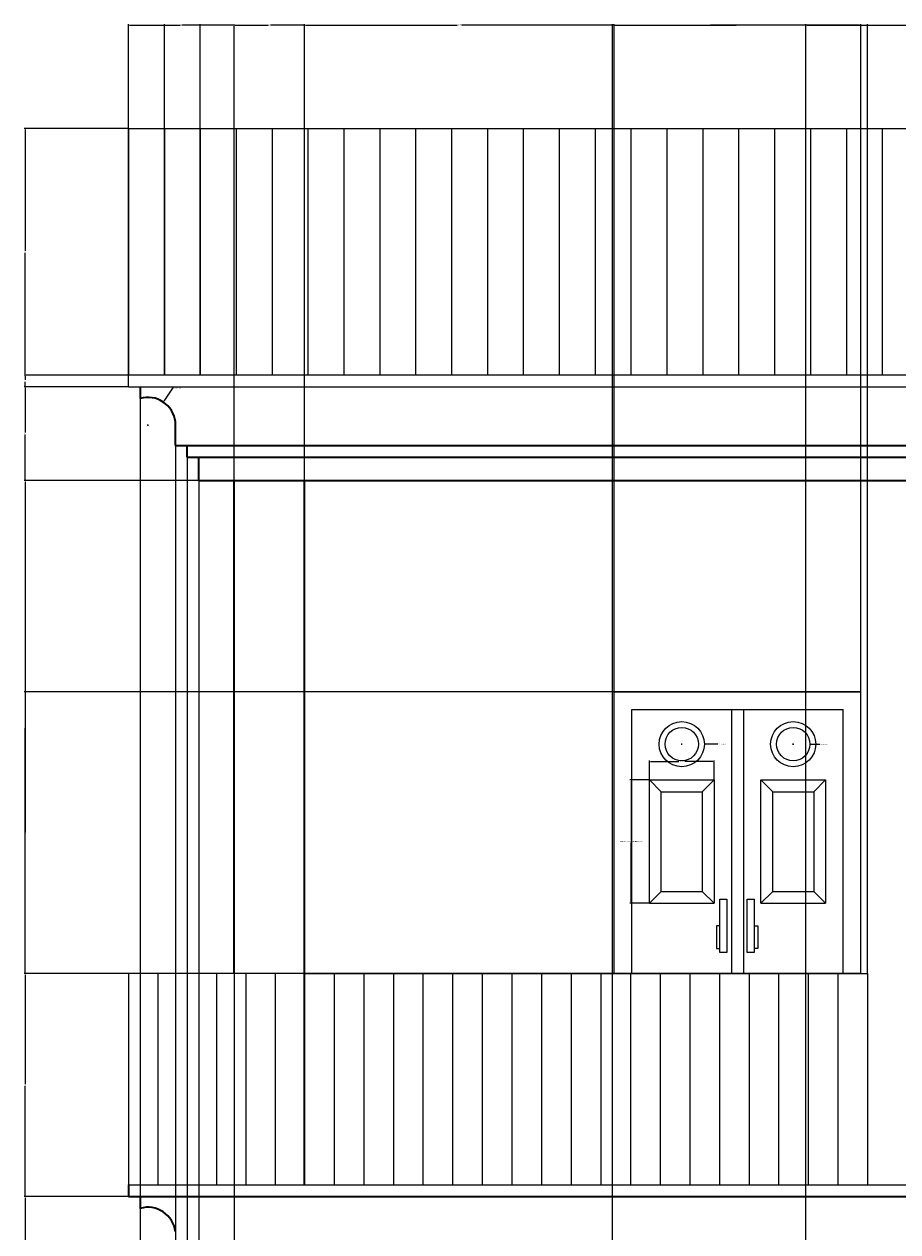
# Model space of a CAD drawing. Units: inches. Extents: x 2612 to 2948, y 481 to 865.
# Tile 5 of 7: x 2613 to 2761, y 659 to 865. Entities that reach past the tile are written whole.
import ezdxf

# ---------------------------------------------------------------- set-up
doc = ezdxf.new("R2010")
doc.units = ezdxf.units.IN
for name, color, linetype, lineweight in [('A-ANNO-DIMS', 2, 'Continuous', 18), ('A-COLS', 1, 'Continuous', 35), ('A-DOOR', 4, 'Continuous', 25), ('A-ELEV', 7, 'Continuous', 35), ('A-ELEV-RAIL', 3, 'Continuous', 18), ('A-ROOF', 7, 'Continuous', 25)]:
    doc.layers.add(name, color=color, linetype=linetype, lineweight=lineweight)
doc.styles.get("Standard").update_dxf_attribs({"font": 'arial.ttf'})
doc.dimstyles.get("Standard").update_dxf_attribs({"dimtxt": 0.18, "dimasz": 0.18, "dimexe": 0.18, "dimexo": 0.0625, "dimgap": 0.09, "dimtad": 0, "dimtih": 1, "dimtoh": 1, "dimdec": 4, "dimzin": 0, "dimdsep": 46, "dimtxsty": 'Standard', "dimcen": 0.09, "dimadec": 0, "dimazin": 0, "dimtfac": 1, "dimtdec": 4, "dimtofl": 0, "dimtmove": 0, "dimatfit": 3, "dimfxl": 1, "dimtolj": 1, "dimtzin": 0, "dimarcsym": 0})

# ---------------------------------------------------------------- blocks, each defined once
blk = doc.blocks.new('DOOR-PANEL-ORNAMENT')
for p, q in [((0, 21), (11, 21)), ((0, 0), (0, 21)), ((2, 19), (0, 21)), ((9, 19), (11, 21)), ((11, 21), (11, 0)), ((2, 2), (2, 19)), ((2, 19), (9, 19)), ((9, 19), (9, 2)), ((2, 2), (0, 0)), ((0, 0), (11, 0)), ((2, 2), (9, 2)), ((9, 2), (11, 0))]:
    blk.add_line(p, q)
blk = doc.blocks.new('*D2')
at = {"layer": 'A-ANNO-DIMS', "color": 0, "lineweight": -2, "transparency": 16777216}
for p, q in [((2719.07, 736.04), (2715.8, 736.04)), ((2715.98, 735.86), (2715.98, 725.73)), ((2715.98, 715.22), (2715.98, 725.36)), ((2719.07, 715.04), (2715.8, 715.04))]:
    blk.add_line(p, q, dxfattribs=at)
at = {"layer": 'A-ANNO-DIMS', "color": 0, "transparency": 16777216}
for points in [[(2715.95, 735.86), (2716.01, 735.86), (2715.98, 736.04)], [(2715.95, 715.22), (2716.01, 715.22), (2715.98, 715.04)]]:
    blk.add_solid(points, dxfattribs=at)
at = {"layer": 'Defpoints', "color": 0, "transparency": 16777216}
for p in [(2715.98, 736.04), (2719.13, 736.04), (2719.13, 715.04)]:
    blk.add_point(p, dxfattribs=at)
at = {"layer": 'A-ANNO-DIMS', "color": 0, "transparency": 16777216, "insert": (2715.98, 725.54), "char_height": 0.18, "attachment_point": 5}
blk.add_mtext('\\A1;DOOR PANEL ORNAMENT 21 TYP.', dxfattribs=at)
blk = doc.blocks.new('*D3')
at = {"layer": 'A-ANNO-DIMS', "color": 0, "lineweight": -2, "transparency": 16777216}
for p, q in [((2719.13, 736.11), (2719.13, 739.37)), ((2719.31, 739.19), (2724.11, 739.19)), ((2729.95, 739.19), (2725.15, 739.19)), ((2730.13, 736.11), (2730.13, 739.37))]:
    blk.add_line(p, q, dxfattribs=at)
at = {"layer": 'A-ANNO-DIMS', "color": 0, "transparency": 16777216}
for points in [[(2719.31, 739.22), (2719.31, 739.16), (2719.13, 739.19)], [(2729.95, 739.22), (2729.95, 739.16), (2730.13, 739.19)]]:
    blk.add_solid(points, dxfattribs=at)
at = {"layer": 'Defpoints', "color": 0, "transparency": 16777216}
for p in [(2730.13, 739.19), (2719.13, 736.04), (2730.13, 736.04)]:
    blk.add_point(p, dxfattribs=at)
at = {"layer": 'A-ANNO-DIMS', "color": 0, "transparency": 16777216, "insert": (2724.63, 739.19), "char_height": 0.18, "attachment_point": 5}
blk.add_mtext('\\A1;11 TYP.', dxfattribs=at)
blk = doc.blocks.new('*D6')
at = {"layer": 'A-ANNO-DIMS', "color": 0, "lineweight": -2, "transparency": 16777216}
for p, q in [((2630.24, 665.04), (2612.53, 665.04)), ((2612.71, 664.86), (2612.71, 657.23)), ((2612.71, 649.22), (2612.71, 656.86)), ((2648.24, 649.04), (2612.53, 649.04))]:
    blk.add_line(p, q, dxfattribs=at)
at = {"layer": 'A-ANNO-DIMS', "color": 0, "transparency": 16777216}
for points in [[(2612.68, 664.86), (2612.74, 664.86), (2612.71, 665.04)], [(2612.68, 649.22), (2612.74, 649.22), (2612.71, 649.04)]]:
    blk.add_solid(points, dxfattribs=at)
at = {"layer": 'Defpoints', "color": 0, "transparency": 16777216}
for p in [(2612.71, 665.04), (2630.31, 665.04), (2648.31, 649.04)]:
    blk.add_point(p, dxfattribs=at)
at = {"layer": 'A-ANNO-DIMS', "color": 0, "transparency": 16777216, "insert": (2612.71, 657.04), "char_height": 0.18, "attachment_point": 5}
blk.add_mtext('\\A1;16', dxfattribs=at)
blk = doc.blocks.new('*D7')
at = {"layer": 'A-ANNO-DIMS', "color": 0, "lineweight": -2, "transparency": 16777216}
for p, q in [((2630.24, 703.04), (2612.53, 703.04)), ((2612.71, 702.86), (2612.71, 684.23)), ((2612.71, 665.22), (2612.71, 683.86)), ((2630.24, 665.04), (2612.53, 665.04))]:
    blk.add_line(p, q, dxfattribs=at)
at = {"layer": 'A-ANNO-DIMS', "color": 0, "transparency": 16777216}
for points in [[(2612.68, 702.86), (2612.74, 702.86), (2612.71, 703.04)], [(2612.68, 665.22), (2612.74, 665.22), (2612.71, 665.04)]]:
    blk.add_solid(points, dxfattribs=at)
at = {"layer": 'Defpoints', "color": 0, "transparency": 16777216}
for p in [(2612.71, 703.04), (2630.31, 703.04), (2630.31, 665.04)]:
    blk.add_point(p, dxfattribs=at)
at = {"layer": 'A-ANNO-DIMS', "color": 0, "transparency": 16777216, "insert": (2612.71, 684.04), "char_height": 0.18, "attachment_point": 5}
blk.add_mtext('\\A1;38', dxfattribs=at)
blk = doc.blocks.new('*D8')
at = {"layer": 'A-ANNO-DIMS', "color": 0, "lineweight": -2, "transparency": 16777216}
for p, q in [((2648.24, 787.04), (2612.53, 787.04)), ((2612.71, 786.86), (2612.71, 745.23)), ((2612.71, 703.22), (2612.71, 744.86)), ((2630.24, 703.04), (2612.53, 703.04))]:
    blk.add_line(p, q, dxfattribs=at)
at = {"layer": 'A-ANNO-DIMS', "color": 0, "transparency": 16777216}
for points in [[(2612.68, 786.86), (2612.74, 786.86), (2612.71, 787.04)], [(2612.68, 703.22), (2612.74, 703.22), (2612.71, 703.04)]]:
    blk.add_solid(points, dxfattribs=at)
at = {"layer": 'Defpoints', "color": 0, "transparency": 16777216}
for p in [(2612.71, 787.04), (2648.31, 787.04), (2630.31, 703.04)]:
    blk.add_point(p, dxfattribs=at)
at = {"layer": 'A-ANNO-DIMS', "color": 0, "transparency": 16777216, "insert": (2612.71, 745.04), "char_height": 0.18, "attachment_point": 5}
blk.add_mtext('\\A1;84', dxfattribs=at)
blk = doc.blocks.new('*D9')
at = {"layer": 'A-ANNO-DIMS', "color": 0, "lineweight": -2, "transparency": 16777216}
for p, q in [((2630.24, 803.04), (2612.53, 803.04)), ((2612.71, 802.86), (2612.71, 795.23)), ((2612.71, 787.22), (2612.71, 794.86)), ((2648.24, 787.04), (2612.53, 787.04))]:
    blk.add_line(p, q, dxfattribs=at)
at = {"layer": 'A-ANNO-DIMS', "color": 0, "transparency": 16777216}
for points in [[(2612.68, 802.86), (2612.74, 802.86), (2612.71, 803.04)], [(2612.68, 787.22), (2612.74, 787.22), (2612.71, 787.04)]]:
    blk.add_solid(points, dxfattribs=at)
at = {"layer": 'Defpoints', "color": 0, "transparency": 16777216}
for p in [(2612.71, 803.04), (2630.31, 803.04), (2648.31, 787.04)]:
    blk.add_point(p, dxfattribs=at)
at = {"layer": 'A-ANNO-DIMS', "color": 0, "transparency": 16777216, "insert": (2612.71, 795.04), "char_height": 0.18, "attachment_point": 5}
blk.add_mtext('\\A1;16', dxfattribs=at)
blk = doc.blocks.new('*D10')
at = {"layer": 'A-ANNO-DIMS', "color": 0, "lineweight": -2, "transparency": 16777216}
for p, q in [((2630.24, 805.04), (2612.53, 805.04)), ((2612.71, 804.86), (2612.71, 804.22)), ((2630.24, 803.04), (2612.53, 803.04)), ((2612.71, 803.22), (2612.71, 803.86))]:
    blk.add_line(p, q, dxfattribs=at)
at = {"layer": 'A-ANNO-DIMS', "color": 0, "transparency": 16777216}
for points in [[(2612.68, 804.86), (2612.74, 804.86), (2612.71, 805.04)], [(2612.68, 803.22), (2612.74, 803.22), (2612.71, 803.04)]]:
    blk.add_solid(points, dxfattribs=at)
at = {"layer": 'Defpoints', "color": 0, "transparency": 16777216}
for p in [(2612.71, 805.04), (2630.31, 805.04), (2630.31, 803.04)]:
    blk.add_point(p, dxfattribs=at)
at = {"layer": 'A-ANNO-DIMS', "color": 0, "transparency": 16777216, "insert": (2612.71, 804.04), "char_height": 0.18, "attachment_point": 5}
blk.add_mtext('\\A1;2', dxfattribs=at)
blk = doc.blocks.new('*D11')
at = {"layer": 'A-ANNO-DIMS', "color": 0, "lineweight": -2, "transparency": 16777216}
for p, q in [((2630.24, 847.04), (2612.53, 847.04)), ((2612.71, 846.86), (2612.71, 826.22)), ((2612.71, 805.22), (2612.71, 825.86)), ((2630.24, 805.04), (2612.53, 805.04))]:
    blk.add_line(p, q, dxfattribs=at)
at = {"layer": 'A-ANNO-DIMS', "color": 0, "transparency": 16777216}
for points in [[(2612.68, 846.86), (2612.74, 846.86), (2612.71, 847.04)], [(2612.68, 805.22), (2612.74, 805.22), (2612.71, 805.04)]]:
    blk.add_solid(points, dxfattribs=at)
at = {"layer": 'Defpoints', "color": 0, "transparency": 16777216}
for p in [(2612.71, 847.04), (2630.31, 847.04), (2630.31, 805.04)]:
    blk.add_point(p, dxfattribs=at)
at = {"layer": 'A-ANNO-DIMS', "color": 0, "transparency": 16777216, "insert": (2612.71, 826.04), "char_height": 0.18, "attachment_point": 5}
blk.add_mtext('\\A1;42', dxfattribs=at)
blk = doc.blocks.new('*D28')
at = {"layer": 'A-ANNO-DIMS', "color": 0, "lineweight": -2, "transparency": 16777216}
for p, q in [((2630.31, 847.11), (2630.31, 864.82)), ((2630.49, 864.64), (2639.1, 864.64)), ((2648.13, 864.64), (2639.52, 864.64)), ((2648.31, 787.11), (2648.31, 864.82))]:
    blk.add_line(p, q, dxfattribs=at)
at = {"layer": 'A-ANNO-DIMS', "color": 0, "transparency": 16777216}
for points in [[(2630.49, 864.67), (2630.49, 864.61), (2630.31, 864.64)], [(2648.13, 864.67), (2648.13, 864.61), (2648.31, 864.64)]]:
    blk.add_solid(points, dxfattribs=at)
at = {"layer": 'Defpoints', "color": 0, "transparency": 16777216}
for p in [(2648.31, 864.64), (2630.31, 847.04), (2648.31, 787.04)]:
    blk.add_point(p, dxfattribs=at)
at = {"layer": 'A-ANNO-DIMS', "color": 0, "transparency": 16777216, "insert": (2639.31, 864.64), "char_height": 0.18, "attachment_point": 5}
blk.add_mtext('\\A1;18', dxfattribs=at)
blk = doc.blocks.new('*D29')
at = {"layer": 'A-ANNO-DIMS', "color": 0, "lineweight": -2, "transparency": 16777216}
for p, q in [((2648.31, 787.11), (2648.31, 864.82)), ((2648.49, 864.64), (2654.1, 864.64)), ((2660.13, 864.64), (2654.52, 864.64)), ((2660.31, 787.11), (2660.31, 864.82))]:
    blk.add_line(p, q, dxfattribs=at)
at = {"layer": 'A-ANNO-DIMS', "color": 0, "transparency": 16777216}
for points in [[(2648.49, 864.67), (2648.49, 864.61), (2648.31, 864.64)], [(2660.13, 864.67), (2660.13, 864.61), (2660.31, 864.64)]]:
    blk.add_solid(points, dxfattribs=at)
at = {"layer": 'Defpoints', "color": 0, "transparency": 16777216}
for p in [(2660.31, 864.64), (2648.31, 787.04), (2660.31, 787.04)]:
    blk.add_point(p, dxfattribs=at)
at = {"layer": 'A-ANNO-DIMS', "color": 0, "transparency": 16777216, "insert": (2654.31, 864.64), "char_height": 0.18, "attachment_point": 5}
blk.add_mtext('\\A1;12', dxfattribs=at)
blk = doc.blocks.new('*D30')
at = {"layer": 'A-ANNO-DIMS', "color": 0, "lineweight": -2, "transparency": 16777216}
for p, q in [((2660.31, 787.11), (2660.31, 864.82)), ((2660.49, 864.64), (2686.33, 864.64)), ((2712.95, 864.64), (2687.11, 864.64)), ((2713.13, 751.11), (2713.13, 864.82))]:
    blk.add_line(p, q, dxfattribs=at)
at = {"layer": 'A-ANNO-DIMS', "color": 0, "transparency": 16777216}
for points in [[(2660.49, 864.67), (2660.49, 864.61), (2660.31, 864.64)], [(2712.95, 864.67), (2712.95, 864.61), (2713.13, 864.64)]]:
    blk.add_solid(points, dxfattribs=at)
at = {"layer": 'Defpoints', "color": 0, "transparency": 16777216}
for p in [(2713.13, 864.64), (2660.31, 787.04), (2713.13, 751.04)]:
    blk.add_point(p, dxfattribs=at)
at = {"layer": 'A-ANNO-DIMS', "color": 0, "transparency": 16777216, "insert": (2686.72, 864.64), "char_height": 0.18, "attachment_point": 5}
blk.add_mtext('\\A1;52.82', dxfattribs=at)
blk = doc.blocks.new('*D31')
at = {"layer": 'A-ANNO-DIMS', "color": 0, "lineweight": -2, "transparency": 16777216}
for p, q in [((2713.13, 751.11), (2713.13, 864.82)), ((2713.31, 864.64), (2733.91, 864.64)), ((2754.95, 864.64), (2734.35, 864.64)), ((2755.13, 751.11), (2755.13, 864.82))]:
    blk.add_line(p, q, dxfattribs=at)
at = {"layer": 'A-ANNO-DIMS', "color": 0, "transparency": 16777216}
for points in [[(2713.31, 864.67), (2713.31, 864.61), (2713.13, 864.64)], [(2754.95, 864.67), (2754.95, 864.61), (2755.13, 864.64)]]:
    blk.add_solid(points, dxfattribs=at)
at = {"layer": 'Defpoints', "color": 0, "transparency": 16777216}
for p in [(2755.13, 864.64), (2713.13, 751.04), (2755.13, 751.04)]:
    blk.add_point(p, dxfattribs=at)
at = {"layer": 'A-ANNO-DIMS', "color": 0, "transparency": 16777216, "insert": (2734.13, 864.64), "char_height": 0.18, "attachment_point": 5}
blk.add_mtext('\\A1;42', dxfattribs=at)
blk = doc.blocks.new('*D32')
at = {"layer": 'A-ANNO-DIMS', "color": 0, "lineweight": -2, "transparency": 16777216}
for p, q in [((2754.95, 864.64), (2754.77, 864.64)), ((2755.13, 751.11), (2755.13, 864.82)), ((2756.31, 703.11), (2756.31, 864.82)), ((2756.49, 864.64), (2756.67, 864.64))]:
    blk.add_line(p, q, dxfattribs=at)
at = {"layer": 'A-ANNO-DIMS', "color": 0, "transparency": 16777216}
for points in [[(2754.95, 864.67), (2754.95, 864.61), (2755.13, 864.64)], [(2756.49, 864.67), (2756.49, 864.61), (2756.31, 864.64)]]:
    blk.add_solid(points, dxfattribs=at)
at = {"layer": 'Defpoints', "color": 0, "transparency": 16777216}
for p in [(2756.31, 864.64), (2755.13, 751.04), (2756.31, 703.04)]:
    blk.add_point(p, dxfattribs=at)
at = {"layer": 'A-ANNO-DIMS', "color": 0, "transparency": 16777216, "insert": (2755.72, 864.64), "char_height": 0.18, "attachment_point": 5}
blk.add_mtext('\\A1;1.177', dxfattribs=at)
blk = doc.blocks.new('*D33')
at = {"layer": 'A-ANNO-DIMS', "color": 0, "lineweight": -2, "transparency": 16777216}
for p, q in [((2756.31, 703.11), (2756.31, 864.82)), ((2756.49, 864.64), (2780.08, 864.64)), ((2804.13, 864.64), (2780.53, 864.64)), ((2804.31, 703.11), (2804.31, 864.82))]:
    blk.add_line(p, q, dxfattribs=at)
at = {"layer": 'A-ANNO-DIMS', "color": 0, "transparency": 16777216}
for points in [[(2756.49, 864.67), (2756.49, 864.61), (2756.31, 864.64)], [(2804.13, 864.67), (2804.13, 864.61), (2804.31, 864.64)]]:
    blk.add_solid(points, dxfattribs=at)
at = {"layer": 'Defpoints', "color": 0, "transparency": 16777216}
for p in [(2804.31, 864.64), (2756.31, 703.04), (2804.31, 703.04)]:
    blk.add_point(p, dxfattribs=at)
at = {"layer": 'A-ANNO-DIMS', "color": 0, "transparency": 16777216, "insert": (2780.31, 864.64), "char_height": 0.18, "attachment_point": 5}
blk.add_mtext('\\A1;48', dxfattribs=at)
blk = doc.blocks.new('*D40')
at = {"layer": 'A-ANNO-DIMS', "color": 0, "lineweight": -2, "transparency": 16777216}
for p, q in [((2755.07, 751.04), (2612.53, 751.04)), ((2612.71, 750.86), (2612.71, 727.23)), ((2612.71, 703.22), (2612.71, 726.86)), ((2755.07, 703.04), (2612.53, 703.04))]:
    blk.add_line(p, q, dxfattribs=at)
at = {"layer": 'A-ANNO-DIMS', "color": 0, "transparency": 16777216}
for points in [[(2612.68, 750.86), (2612.74, 750.86), (2612.71, 751.04)], [(2612.68, 703.22), (2612.74, 703.22), (2612.71, 703.04)]]:
    blk.add_solid(points, dxfattribs=at)
at = {"layer": 'Defpoints', "color": 0, "transparency": 16777216}
for p in [(2755.13, 751.04), (2612.71, 703.04), (2755.13, 703.04)]:
    blk.add_point(p, dxfattribs=at)
at = {"layer": 'A-ANNO-DIMS', "color": 0, "transparency": 16777216, "insert": (2612.71, 727.04), "char_height": 0.18, "attachment_point": 5}
blk.add_mtext('\\A1;48', dxfattribs=at)
blk = doc.blocks.new('*D41')
at = {"layer": 'A-ANNO-DIMS', "color": 0, "lineweight": -2, "transparency": 16777216}
for p, q in [((2632.31, 802.98), (2632.31, 481.26)), ((2638.31, 792.98), (2638.31, 481.26)), ((2632.49, 481.44), (2635.16, 481.44)), ((2638.13, 481.44), (2635.46, 481.44))]:
    blk.add_line(p, q, dxfattribs=at)
at = {"layer": 'A-ANNO-DIMS', "color": 0, "transparency": 16777216}
for points in [[(2632.49, 481.47), (2632.49, 481.41), (2632.31, 481.44)], [(2638.13, 481.47), (2638.13, 481.41), (2638.31, 481.44)]]:
    blk.add_solid(points, dxfattribs=at)
at = {"layer": 'Defpoints', "color": 0, "transparency": 16777216}
for p in [(2632.31, 803.04), (2638.31, 793.04), (2638.31, 481.44)]:
    blk.add_point(p, dxfattribs=at)
at = {"layer": 'A-ANNO-DIMS', "color": 0, "transparency": 16777216, "insert": (2635.31, 481.44), "char_height": 0.18, "attachment_point": 5}
blk.add_mtext('\\A1;6', dxfattribs=at)
blk = doc.blocks.new('*D42')
at = {"layer": 'A-ANNO-DIMS', "color": 0, "lineweight": -2, "transparency": 16777216}
for p, q in [((2638.31, 792.98), (2638.31, 481.26)), ((2640.31, 790.98), (2640.31, 481.26)), ((2638.49, 481.44), (2639.16, 481.44)), ((2640.13, 481.44), (2639.46, 481.44))]:
    blk.add_line(p, q, dxfattribs=at)
at = {"layer": 'A-ANNO-DIMS', "color": 0, "transparency": 16777216}
for points in [[(2638.49, 481.47), (2638.49, 481.41), (2638.31, 481.44)], [(2640.13, 481.47), (2640.13, 481.41), (2640.31, 481.44)]]:
    blk.add_solid(points, dxfattribs=at)
at = {"layer": 'Defpoints', "color": 0, "transparency": 16777216}
for p in [(2638.31, 793.04), (2640.31, 791.04), (2640.31, 481.44)]:
    blk.add_point(p, dxfattribs=at)
at = {"layer": 'A-ANNO-DIMS', "color": 0, "transparency": 16777216, "insert": (2639.31, 481.44), "char_height": 0.18, "attachment_point": 5}
blk.add_mtext('\\A1;2', dxfattribs=at)
blk = doc.blocks.new('*D43')
at = {"layer": 'A-ANNO-DIMS', "color": 0, "lineweight": -2, "transparency": 16777216}
for p, q in [((2640.31, 790.98), (2640.31, 481.26)), ((2642.31, 786.98), (2642.31, 481.26)), ((2640.49, 481.44), (2641.16, 481.44)), ((2642.13, 481.44), (2641.46, 481.44))]:
    blk.add_line(p, q, dxfattribs=at)
at = {"layer": 'A-ANNO-DIMS', "color": 0, "transparency": 16777216}
for points in [[(2640.49, 481.47), (2640.49, 481.41), (2640.31, 481.44)], [(2642.13, 481.47), (2642.13, 481.41), (2642.31, 481.44)]]:
    blk.add_solid(points, dxfattribs=at)
at = {"layer": 'Defpoints', "color": 0, "transparency": 16777216}
for p in [(2640.31, 791.04), (2642.31, 787.04), (2642.31, 481.44)]:
    blk.add_point(p, dxfattribs=at)
at = {"layer": 'A-ANNO-DIMS', "color": 0, "transparency": 16777216, "insert": (2641.31, 481.44), "char_height": 0.18, "attachment_point": 5}
blk.add_mtext('\\A1;2', dxfattribs=at)
blk = doc.blocks.new('*D44')
at = {"layer": 'A-ANNO-DIMS', "color": 0, "lineweight": -2, "transparency": 16777216}
for p, q in [((2642.31, 786.98), (2642.31, 481.26)), ((2648.31, 786.98), (2648.31, 481.26)), ((2642.49, 481.44), (2645.16, 481.44)), ((2648.13, 481.44), (2645.46, 481.44))]:
    blk.add_line(p, q, dxfattribs=at)
at = {"layer": 'A-ANNO-DIMS', "color": 0, "transparency": 16777216}
for points in [[(2642.49, 481.47), (2642.49, 481.41), (2642.31, 481.44)], [(2648.13, 481.47), (2648.13, 481.41), (2648.31, 481.44)]]:
    blk.add_solid(points, dxfattribs=at)
at = {"layer": 'Defpoints', "color": 0, "transparency": 16777216}
for p in [(2642.31, 787.04), (2648.31, 787.04), (2648.31, 481.44)]:
    blk.add_point(p, dxfattribs=at)
at = {"layer": 'A-ANNO-DIMS', "color": 0, "transparency": 16777216, "insert": (2645.31, 481.44), "char_height": 0.18, "attachment_point": 5}
blk.add_mtext('\\A1;6', dxfattribs=at)
blk = doc.blocks.new('*D45')
at = {"layer": 'A-ANNO-DIMS', "color": 0, "lineweight": -2, "transparency": 16777216}
for p, q in [((2640.369922, 791.044274), (2948.087422, 791.044274)), ((2947.907422, 790.864274), (2947.907422, 789.224274)), ((2947.907422, 787.224274), (2947.907422, 788.864274)), ((2642.369922, 787.044274), (2948.087422, 787.044274))]:
    blk.add_line(p, q, dxfattribs=at)
at = {"layer": 'A-ANNO-DIMS', "color": 0, "transparency": 16777216}
for points in [[(2947.877422, 790.864274), (2947.937422, 790.864274), (2947.907422, 791.044274)], [(2947.877422, 787.224274), (2947.937422, 787.224274), (2947.907422, 787.044274)]]:
    blk.add_solid(points, dxfattribs=at)
at = {"layer": 'Defpoints', "color": 0, "transparency": 16777216}
for p in [(2640.307422, 791.044274), (2947.907422, 791.044274), (2642.307422, 787.044274)]:
    blk.add_point(p, dxfattribs=at)
at = {"layer": 'A-ANNO-DIMS', "color": 0, "transparency": 16777216, "insert": (2947.907422, 789.044274), "char_height": 0.18, "attachment_point": 5}
blk.add_mtext('\\A1;4', dxfattribs=at)
blk = doc.blocks.new('*D46')
at = {"layer": 'A-ANNO-DIMS', "color": 0, "lineweight": -2, "transparency": 16777216}
for p, q in [((2638.37, 793.04), (2948.09, 793.04)), ((2947.91, 792.86), (2947.91, 792.22)), ((2640.37, 791.04), (2948.09, 791.04)), ((2947.91, 791.22), (2947.91, 791.86))]:
    blk.add_line(p, q, dxfattribs=at)
at = {"layer": 'A-ANNO-DIMS', "color": 0, "transparency": 16777216}
for points in [[(2947.88, 792.86), (2947.94, 792.86), (2947.91, 793.04)], [(2947.88, 791.22), (2947.94, 791.22), (2947.91, 791.04)]]:
    blk.add_solid(points, dxfattribs=at)
at = {"layer": 'Defpoints', "color": 0, "transparency": 16777216}
for p in [(2638.31, 793.04), (2947.91, 793.04), (2640.31, 791.04)]:
    blk.add_point(p, dxfattribs=at)
at = {"layer": 'A-ANNO-DIMS', "color": 0, "transparency": 16777216, "insert": (2947.91, 792.04), "char_height": 0.18, "attachment_point": 5}
blk.add_mtext('\\A1;2', dxfattribs=at)
blk = doc.blocks.new('*D47')
at = {"layer": 'A-ANNO-DIMS', "color": 0, "lineweight": -2, "transparency": 16777216}
for p, q in [((2632.37, 803.04), (2948.09, 803.04)), ((2947.91, 802.86), (2947.91, 798.23)), ((2947.91, 793.22), (2947.91, 797.86)), ((2638.37, 793.04), (2948.09, 793.04))]:
    blk.add_line(p, q, dxfattribs=at)
at = {"layer": 'A-ANNO-DIMS', "color": 0, "transparency": 16777216}
for points in [[(2947.88, 802.86), (2947.94, 802.86), (2947.91, 803.04)], [(2947.88, 793.22), (2947.94, 793.22), (2947.91, 793.04)]]:
    blk.add_solid(points, dxfattribs=at)
at = {"layer": 'Defpoints', "color": 0, "transparency": 16777216}
for p in [(2632.31, 803.04), (2947.91, 803.04), (2638.31, 793.04)]:
    blk.add_point(p, dxfattribs=at)
at = {"layer": 'A-ANNO-DIMS', "color": 0, "transparency": 16777216, "insert": (2947.91, 798.04), "char_height": 0.18, "attachment_point": 5}
blk.add_mtext('\\A1;10', dxfattribs=at)
blk = doc.blocks.new('*D48')
at = {"layer": 'A-ANNO-DIMS', "color": 0, "lineweight": -2, "transparency": 16777216}
for p, q in [((2636.43, 805.11), (2636.43, 864.82)), ((2636.61, 864.64), (2639.09, 864.64)), ((2642.37, 864.64), (2639.88, 864.64)), ((2642.55, 805.11), (2642.55, 864.82))]:
    blk.add_line(p, q, dxfattribs=at)
at = {"layer": 'A-ANNO-DIMS', "color": 0, "transparency": 16777216}
for points in [[(2636.61, 864.67), (2636.61, 864.61), (2636.43, 864.64)], [(2642.37, 864.67), (2642.37, 864.61), (2642.55, 864.64)]]:
    blk.add_solid(points, dxfattribs=at)
at = {"layer": 'Defpoints', "color": 0, "transparency": 16777216}
for p in [(2642.55, 864.64), (2636.43, 805.04), (2642.55, 805.04)]:
    blk.add_point(p, dxfattribs=at)
at = {"layer": 'A-ANNO-DIMS', "color": 0, "transparency": 16777216, "insert": (2639.49, 864.64), "char_height": 0.18, "attachment_point": 5}
blk.add_mtext('\\A1;6.119', dxfattribs=at)
blk = doc.blocks.new('*D49')
at = {"layer": 'A-ANNO-DIMS', "color": 0, "lineweight": -2, "transparency": 16777216}
for p, q in [((2712.81, 562.11), (2712.81, 864.82)), ((2712.99, 864.64), (2729.09, 864.64)), ((2745.63, 864.64), (2729.53, 864.64)), ((2745.81, 604.11), (2745.81, 864.82))]:
    blk.add_line(p, q, dxfattribs=at)
at = {"layer": 'A-ANNO-DIMS', "color": 0, "transparency": 16777216}
for points in [[(2712.99, 864.67), (2712.99, 864.61), (2712.81, 864.64)], [(2745.63, 864.67), (2745.63, 864.61), (2745.81, 864.64)]]:
    blk.add_solid(points, dxfattribs=at)
at = {"layer": 'Defpoints', "color": 0, "transparency": 16777216}
for p in [(2745.81, 864.64), (2745.81, 604.04), (2712.81, 562.04)]:
    blk.add_point(p, dxfattribs=at)
at = {"layer": 'A-ANNO-DIMS', "color": 0, "transparency": 16777216, "insert": (2729.31, 864.64), "char_height": 0.18, "attachment_point": 5}
blk.add_mtext('\\A1;33', dxfattribs=at)
blk = doc.blocks.new('*D50')
at = {"layer": 'A-ANNO-DIMS', "color": 0, "lineweight": -2, "transparency": 16777216}
for p, q in [((2745.81, 604.11), (2745.81, 864.82)), ((2745.99, 864.64), (2769.58, 864.64)), ((2793.63, 864.64), (2770.03, 864.64)), ((2793.81, 604.11), (2793.81, 864.82))]:
    blk.add_line(p, q, dxfattribs=at)
at = {"layer": 'A-ANNO-DIMS', "color": 0, "transparency": 16777216}
for points in [[(2745.99, 864.67), (2745.99, 864.61), (2745.81, 864.64)], [(2793.63, 864.67), (2793.63, 864.61), (2793.81, 864.64)]]:
    blk.add_solid(points, dxfattribs=at)
at = {"layer": 'Defpoints', "color": 0, "transparency": 16777216}
for p in [(2793.81, 864.64), (2745.81, 604.04), (2793.81, 604.04)]:
    blk.add_point(p, dxfattribs=at)
at = {"layer": 'A-ANNO-DIMS', "color": 0, "transparency": 16777216, "insert": (2769.81, 864.64), "char_height": 0.18, "attachment_point": 5}
blk.add_mtext('\\A1;48', dxfattribs=at)
blk = doc.blocks.new('*D90')
at = {"layer": 'A-ANNO-DIMS', "color": 0, "lineweight": -2, "transparency": 16777216}
for p, q in [((2724.54, 742.14), (2724.72, 742.14)), ((2724.63, 742.05), (2724.63, 742.23)), ((2730.79, 742.14), (2728.66, 742.14))]:
    blk.add_line(p, q, dxfattribs=at)
at = {"layer": 'A-ANNO-DIMS', "color": 0, "transparency": 16777216}
blk.add_solid([(2728.66, 742.17), (2728.66, 742.11), (2728.48, 742.14)], dxfattribs=at)
at = {"layer": 'Defpoints', "color": 0, "transparency": 16777216}
for p in [(2720.78, 742.14), (2728.48, 742.14)]:
    blk.add_point(p, dxfattribs=at)
at = {"layer": 'A-ANNO-DIMS', "color": 0, "transparency": 16777216, "insert": (2731.47, 742.14), "char_height": 0.18, "attachment_point": 5}
blk.add_mtext('\\A1;2X ∅7.699', dxfattribs=at)
blk = doc.blocks.new('*D91')
at = {"layer": 'A-ANNO-DIMS', "color": 0, "lineweight": -2, "transparency": 16777216}
for p, q in [((2743.54, 742.14), (2743.72, 742.14)), ((2743.63, 742.05), (2743.63, 742.23)), ((2748.19, 742.07), (2746.66, 742.1))]:
    blk.add_line(p, q, dxfattribs=at)
at = {"layer": 'A-ANNO-DIMS', "color": 0, "transparency": 16777216}
blk.add_solid([(2746.66, 742.13), (2746.66, 742.07), (2746.48, 742.1)], dxfattribs=at)
at = {"layer": 'Defpoints', "color": 0, "transparency": 16777216}
for p in [(2740.78, 742.19), (2746.48, 742.1)]:
    blk.add_point(p, dxfattribs=at)
at = {"layer": 'A-ANNO-DIMS', "color": 0, "transparency": 16777216, "insert": (2748.87, 742.07), "char_height": 0.18, "attachment_point": 5}
blk.add_mtext('\\A1;2X ∅5.699', dxfattribs=at)
blk = doc.blocks.new('*D92')
at = {"layer": 'A-ANNO-DIMS', "color": 0, "lineweight": -2, "transparency": 16777216}
for p, q in [((2637.81, 802.79), (2636.34, 800.59)), ((2637.99, 802.79), (2637.81, 802.79)), ((2633.53, 796.52), (2633.71, 796.52)), ((2633.62, 796.43), (2633.62, 796.61))]:
    blk.add_line(p, q, dxfattribs=at)
at = {"layer": 'A-ANNO-DIMS', "color": 0, "transparency": 16777216}
blk.add_solid([(2636.31, 800.61), (2636.36, 800.57), (2636.24, 800.44)], dxfattribs=at)
at = {"layer": 'Defpoints', "color": 0, "transparency": 16777216}
for p in [(2636.24, 800.44), (2633.62, 796.52)]:
    blk.add_point(p, dxfattribs=at)
at = {"layer": 'A-ANNO-DIMS', "color": 0, "transparency": 16777216, "insert": (2638.66, 802.79), "char_height": 0.18, "attachment_point": 5}
blk.add_mtext('\\A1;4X R4.713', dxfattribs=at)

msp = doc.modelspace()

# ---------------------------------------------------------------- linework, layer by layer
at = {"layer": 'A-COLS'}
for p, q in [((2648.3074, 703.0443), (2648.3074, 787.0443)), ((2660.3074, 667.0443), (2660.3074, 787.0443))]:
    msp.add_line(p, q, dxfattribs=at)
at = {"layer": 'A-DOOR'}
for p, q in [((2713.1304, 703.0443), (2713.1304, 751.0443)), ((2713.1304, 751.0443), (2755.1304, 751.0443)), ((2755.1304, 703.0443), (2755.1304, 751.0443)), ((2716.1304, 748.0443), (2752.1304, 748.0443)), ((2716.1304, 703.0443), (2716.1304, 748.0443)), ((2733.1304, 748.0443), (2733.1304, 703.0443)), ((2735.1304, 748.0443), (2735.1304, 703.0443)), ((2752.1304, 703.0443), (2752.1304, 748.0443))]:
    msp.add_line(p, q, dxfattribs=at)
for points in [[(2731.1038, 715.7089), (2732.2867, 715.7089), (2732.2867, 706.6701), (2731.1038, 706.6701)], [(2735.7764, 715.7089), (2736.9593, 715.7089), (2736.9593, 706.6701), (2735.7764, 706.6701)]]:
    msp.add_lwpolyline(points, close=True, dxfattribs=at)
for points in [[(2731.1038, 711.1895), (2730.5459, 711.1895), (2730.5459, 707.3195), (2731.1038, 707.3195)], [(2736.9593, 711.1895), (2737.5762, 711.1895), (2737.5762, 707.3195), (2736.9593, 707.3195)]]:
    msp.add_lwpolyline(points, dxfattribs=at)
for centre, radius in [((2724.6304, 742.143), 3.8494), ((2724.6304, 742.143), 2.8494), ((2743.6304, 742.143), 3.8494), ((2743.6304, 742.143), 2.8494)]:
    msp.add_circle(centre, radius, dxfattribs=at)
at = {"layer": 'A-ELEV'}
for p, q in [((2632.3074, 803.0443), (2632.3074, 801.0443)), ((2638.3074, 793.0443), (2638.3074, 797.0443)), ((2638.3074, 793.0443), (2922.3074, 793.0443)), ((2640.3074, 791.0443), (2640.3074, 793.0443)), ((2640.3074, 791.0443), (2920.3074, 791.0443)), ((2642.3074, 787.0443), (2642.3074, 791.0443)), ((2642.3074, 787.0443), (2918.3074, 787.0443)), ((2630.3074, 667.0443), (2630.3074, 665.0443)), ((2630.3074, 665.0443), (2930.3074, 665.0443)), ((2630.3074, 665.0443), (2632.3074, 665.0443)), ((2632.3074, 665.0443), (2637.3074, 665.0443)), ((2632.3074, 665.0443), (2632.3074, 663.0443))]:
    msp.add_line(p, q, dxfattribs=at)
for centre in [(2633.6239, 796.519), (2633.6239, 658.519)]:
    msp.add_arc(centre, 4.7129, 6.399265, 106.2206, dxfattribs=at)
at = {"layer": 'A-ELEV-RAIL'}
for p, q in [((2660.3074, 703.0443), (2630.3074, 703.0443)), ((2630.3074, 703.0443), (2630.3074, 667.0443)), ((2635.3074, 703.0443), (2635.3074, 667.0443)), ((2640.3074, 703.0443), (2640.3074, 667.0443)), ((2645.3074, 703.0443), (2645.3074, 667.0443)), ((2650.3074, 703.0443), (2650.3074, 667.0443)), ((2655.3074, 703.0443), (2655.3074, 667.0443)), ((2660.3074, 703.0443), (2756.3074, 703.0443)), ((2660.3074, 703.0443), (2660.3074, 667.0443)), ((2665.3601, 703.0443), (2665.3601, 667.0443)), ((2670.4127, 703.0443), (2670.4127, 667.0443)), ((2675.4653, 703.0443), (2675.4653, 667.0443)), ((2680.5179, 703.0443), (2680.5179, 667.0443)), ((2685.5706, 703.0443), (2685.5706, 667.0443)), ((2690.6232, 703.0443), (2690.6232, 667.0443)), ((2695.6758, 703.0443), (2695.6758, 667.0443)), ((2700.7285, 703.0443), (2700.7285, 667.0443)), ((2705.7811, 703.0443), (2705.7811, 667.0443)), ((2710.8337, 703.0443), (2710.8337, 667.0443)), ((2715.8864, 703.0443), (2715.8864, 667.0443)), ((2720.939, 703.0443), (2720.939, 667.0443)), ((2725.9916, 703.0443), (2725.9916, 667.0443)), ((2731.0443, 703.0443), (2731.0443, 667.0443)), ((2736.0969, 703.0443), (2736.0969, 667.0443)), ((2741.1495, 703.0443), (2741.1495, 667.0443)), ((2746.2022, 703.0443), (2746.2022, 667.0443)), ((2751.2548, 703.0443), (2751.2548, 667.0443)), ((2756.3074, 703.0443), (2756.3074, 667.0443)), ((2630.3074, 667.0443), (2930.3074, 667.0443))]:
    msp.add_line(p, q, dxfattribs=at)
at = {"layer": 'A-ROOF'}
for p, q in [((2630.3074, 847.0443), (2930.3074, 847.0443)), ((2630.3074, 803.0443), (2630.3074, 847.0443)), ((2630.3074, 847.0443), (2630.3074, 805.0443)), ((2636.4265, 847.0443), (2636.4265, 805.0443)), ((2642.5456, 847.0443), (2642.5456, 805.0443)), ((2648.6647, 847.0443), (2648.6647, 805.0443)), ((2654.7839, 847.0443), (2654.7839, 805.0443)), ((2660.903, 847.0443), (2660.903, 805.0443)), ((2667.0221, 847.0443), (2667.0221, 805.0443)), ((2673.1412, 847.0443), (2673.1412, 805.0443)), ((2679.2603, 847.0443), (2679.2603, 805.0443)), ((2685.3794, 847.0443), (2685.3794, 805.0443)), ((2691.4985, 847.0443), (2691.4985, 805.0443)), ((2697.6176, 847.0443), (2697.6176, 805.0443)), ((2703.7367, 847.0443), (2703.7367, 805.0443)), ((2709.8558, 847.0443), (2709.8558, 805.0443)), ((2715.9749, 847.0443), (2715.9749, 805.0443)), ((2722.094, 847.0443), (2722.094, 805.0443)), ((2728.2132, 847.0443), (2728.2132, 805.0443)), ((2734.3323, 847.0443), (2734.3323, 805.0443)), ((2740.4514, 847.0443), (2740.4514, 805.0443)), ((2746.5705, 847.0443), (2746.5705, 805.0443)), ((2752.6896, 847.0443), (2752.6896, 805.0443)), ((2758.8087, 847.0443), (2758.8087, 805.0443)), ((2630.3074, 805.0443), (2930.3074, 805.0443)), ((2630.3074, 803.0443), (2930.3074, 803.0443))]:
    msp.add_line(p, q, dxfattribs=at)

# ---------------------------------------------------------------- block references
at = {"layer": 'A-DOOR'}
for p in [(2719.13, 715.044), (2738.13, 715.044)]:
    msp.add_blockref('DOOR-PANEL-ORNAMENT', p, dxfattribs=at)

# ---------------------------------------------------------------- dimensions: what is measured, and where the dimension line sits
at = {"layer": 'A-ANNO-DIMS'}
for base, p1, p2, override, picture, middle in [((2648.3074, 864.6443), (2630.3074, 847.0443), (2648.3074, 787.0443), {"dimdec": 0, "dimlfac": 1, "dimrnd": 0, "dimzin": 0, "dimdsep": 46, "dimlunit": 2}, '*D28', (2639.3074, 864.6443)), ((2642.5456, 864.6443), (2636.4265, 805.0443), (2642.5456, 805.0443), {"dimdec": 3, "dimlfac": 1, "dimrnd": 0, "dimzin": 0, "dimdsep": 46, "dimlunit": 2}, '*D48', (2639.4861, 864.6443)), ((2660.3074, 864.6443), (2648.3074, 787.0443), (2660.3074, 787.0443), {"dimdec": 0, "dimlfac": 1, "dimrnd": 0, "dimzin": 0, "dimdsep": 46, "dimlunit": 2}, '*D29', (2654.3074, 864.6443)), ((2713.1304, 864.6443), (2660.3074, 787.0443), (2713.1304, 751.0443), {"dimdec": 2, "dimlfac": 1, "dimrnd": 0, "dimzin": 0, "dimdsep": 46, "dimlunit": 2}, '*D30', (2686.7189, 864.6443)), ((2745.8074, 864.6443), (2712.8074, 562.0443), (2745.8074, 604.0443), {"dimdec": 0, "dimlfac": 1, "dimrnd": 0, "dimzin": 0, "dimdsep": 46, "dimlunit": 2}, '*D49', (2729.3074, 864.6443)), ((2755.1304, 864.6443), (2713.1304, 751.0443), (2755.1304, 751.0443), {"dimdec": 0, "dimlfac": 1, "dimrnd": 0, "dimzin": 0, "dimdsep": 46, "dimlunit": 2}, '*D31', (2734.1304, 864.6443)), ((2793.8074, 864.6443), (2745.8074, 604.0443), (2793.8074, 604.0443), {"dimdec": 0, "dimlfac": 1, "dimrnd": 0, "dimzin": 0, "dimdsep": 46, "dimlunit": 2}, '*D50', (2769.8074, 864.6443)), ((2756.3074, 864.6443), (2755.1304, 751.0443), (2756.3074, 703.0443), {"dimdec": 3, "dimlfac": 1, "dimrnd": 0, "dimzin": 0, "dimdsep": 46, "dimlunit": 2}, '*D32', (2755.7189, 864.6443)), ((2804.3074, 864.6443), (2756.3074, 703.0443), (2804.3074, 703.0443), {"dimdec": 0, "dimlfac": 1, "dimrnd": 0, "dimzin": 0, "dimdsep": 46, "dimlunit": 2}, '*D33', (2780.3074, 864.6443)), ((2638.3074, 481.4443), (2632.3074, 803.0443), (2638.3074, 793.0443), {"dimdec": 0, "dimlfac": 1, "dimrnd": 0, "dimzin": 0, "dimdsep": 46, "dimlunit": 2}, '*D41', (2635.3074, 481.4443)), ((2640.3074, 481.4443), (2638.3074, 793.0443), (2640.3074, 791.0443), {"dimdec": 0, "dimlfac": 1, "dimrnd": 0, "dimzin": 0, "dimdsep": 46, "dimlunit": 2}, '*D42', (2639.3074, 481.4443)), ((2642.3074, 481.4443), (2640.3074, 791.0443), (2642.3074, 787.0443), {"dimdec": 0, "dimlfac": 1, "dimrnd": 0, "dimzin": 0, "dimdsep": 46, "dimlunit": 2}, '*D43', (2641.3074, 481.4443)), ((2648.3074, 481.4443), (2642.3074, 787.0443), (2648.3074, 787.0443), {"dimdec": 0, "dimlfac": 1, "dimrnd": 0, "dimzin": 0, "dimdsep": 46, "dimlunit": 2}, '*D44', (2645.3074, 481.4443))]:
    dim = msp.add_linear_dim(base=base, p1=p1, p2=p2, dimstyle='Standard', override=override, dxfattribs=at)
    dim.commit()
    dim.dimension.update_dxf_attribs({"geometry": picture, "text_midpoint": middle})
for base, p1, p2, picture, middle in [((2612.7074, 847.0443), (2630.3074, 805.0443), (2630.3074, 847.0443), '*D11', (2612.7074, 826.0443)), ((2612.7074, 805.0443), (2630.3074, 803.0443), (2630.3074, 805.0443), '*D10', (2612.7074, 804.0443)), ((2612.7074, 803.0443), (2648.3074, 787.0443), (2630.3074, 803.0443), '*D9', (2612.7074, 795.0443)), ((2947.9074, 803.0443), (2638.3074, 793.0443), (2632.3074, 803.0443), '*D47', (2947.9074, 798.0443)), ((2947.9074, 793.0443), (2640.3074, 791.0443), (2638.3074, 793.0443), '*D46', (2947.9074, 792.0443)), ((2947.9074, 791.0443), (2642.3074, 787.0443), (2640.3074, 791.0443), '*D45', (2947.9074, 789.0443)), ((2612.7074, 787.0443), (2630.3074, 703.0443), (2648.3074, 787.0443), '*D8', (2612.7074, 745.0443)), ((2612.7074, 703.0443), (2755.1304, 751.0443), (2755.1304, 703.0443), '*D40', (2612.7074, 727.0443)), ((2612.7074, 703.0443), (2630.3074, 665.0443), (2630.3074, 703.0443), '*D7', (2612.7074, 684.0443)), ((2612.7074, 665.0443), (2648.3074, 649.0443), (2630.3074, 665.0443), '*D6', (2612.7074, 657.0443))]:
    dim = msp.add_linear_dim(base=base, p1=p1, p2=p2, angle=90, dimstyle='Standard', override={"dimdec": 0, "dimlfac": 1, "dimrnd": 0, "dimzin": 0, "dimdsep": 46, "dimlunit": 2}, dxfattribs=at)
    dim.commit()
    dim.dimension.update_dxf_attribs({"geometry": picture, "text_midpoint": middle})
dim = msp.add_radius_dim(center=(2633.6239, 796.519), mpoint=(2636.2382, 800.4403), text='4X <>', dimstyle='Standard', override={"dimdec": 3, "dimlfac": 1, "dimrnd": 0, "dimzin": 0, "dimdsep": 46, "dimlunit": 2}, dxfattribs=at)
dim.commit()
dim.dimension.update_dxf_attribs({"geometry": '*D92', "text_midpoint": (2638.6636, 802.7931), "dimtype": 164})
for p1, p2, picture, middle in [((2720.781, 742.1431), (2728.4798, 742.143), '*D90', (2730.7895, 742.143)), ((2740.7813, 742.1861), (2746.4795, 742.1), '*D91', (2748.189, 742.0742))]:
    dim = msp.add_diameter_dim_2p(p1=p1, p2=p2, text='2X <>', dimstyle='Standard', override={"dimdec": 3, "dimlfac": 1, "dimrnd": 0, "dimzin": 0, "dimdsep": 46, "dimlunit": 2}, dxfattribs=at)
    dim.commit()
    dim.dimension.update_dxf_attribs({"geometry": picture, "text_midpoint": middle, "dimtype": 163})
dim = msp.add_linear_dim(base=(2730.1304, 739.1943), p1=(2719.1304, 736.0443), p2=(2730.1304, 736.0443), text='<> TYP.', dimstyle='Standard', override={"dimdec": 0, "dimrnd": 0, "dimzin": 0, "dimlunit": 2}, dxfattribs=at)
dim.commit()
dim.dimension.update_dxf_attribs({"geometry": '*D3', "text_midpoint": (2724.6304, 739.1943)})
dim = msp.add_linear_dim(base=(2715.9804, 736.0443), p1=(2719.1304, 715.0443), p2=(2719.1304, 736.0443), angle=90, text='DOOR PANEL ORNAMENT <> TYP.', dimstyle='Standard', override={"dimdec": 0, "dimrnd": 0, "dimzin": 0, "dimlunit": 2}, dxfattribs=at)
dim.commit()
dim.dimension.update_dxf_attribs({"geometry": '*D2', "text_midpoint": (2715.9804, 725.5443)})

doc.saveas('drawing.dxf')
